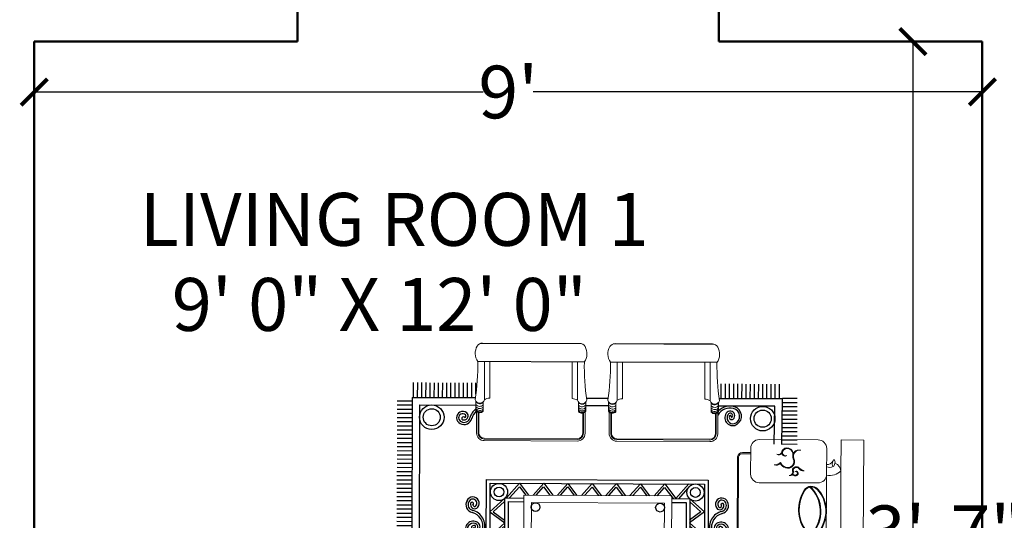
# Model space of a CAD drawing. Units: inches. Extents: x 147 to 1638, y 107 to 941.
# Tile 4 of 17: x 357 to 469, y 341 to 398. Entities that reach past the tile are written whole.
import ezdxf

# ---------------------------------------------------------------- set-up
doc = ezdxf.new("R2010")
doc.units = ezdxf.units.IN
doc.header["$MEASUREMENT"] = 0
for name, color, linetype, lineweight in [('A-ANNO-DIMS', 2, 'Continuous', 15), ('A-AREA-IDEN', 7, 'Continuous', 18), ('furniture', 50, 'Continuous', 18), ('wall', 7, 'Continuous', 60), ('walls', 7, 'Continuous', 50)]:
    doc.layers.add(name, color=color, linetype=linetype, lineweight=lineweight)
doc.layers.add('CARPET', color=40, linetype='Continuous')
doc.styles.get("Standard").update_dxf_attribs({"font": 'arial.ttf'})
doc.dimstyles.get("Standard").update_dxf_attribs({"dimtxt": 6, "dimasz": 3, "dimexe": 0.18, "dimexo": 0.0625, "dimgap": 0.09, "dimtad": 0, "dimtih": 1, "dimtoh": 1, "dimdec": 1, "dimzin": 0, "dimdsep": 46, "dimlunit": 3, "dimtxsty": 'Standard', "dimblk": 'ARCHTICK', "dimcen": 0.09, "dimadec": 0, "dimazin": 0, "dimtfac": 1, "dimtdec": 1, "dimtofl": 0, "dimtmove": 0, "dimatfit": 3, "dimfxl": 1, "dimtolj": 1, "dimtzin": 0, "dimarcsym": 0})

# ---------------------------------------------------------------- blocks, each defined once
blk = doc.blocks.new('_ArchTick')
at = {"color": 0, "linetype": 'ByBlock', "const_width": 0.15}
blk.add_lwpolyline([(-0.5, -0.5), (0.5, 0.5)], dxfattribs=at)
blk = doc.blocks.new('*D30')
at = {"layer": 'A-ANNO-DIMS', "color": 0, "lineweight": -2, "transparency": 16777216}
for p, q in [((460.3, 395.72), (458.86, 395.72)), ((459.04, 395.72), (459.04, 326.82)), ((459.04, 251.72), (459.04, 320.62)), ((460.3, 251.72), (458.86, 251.72))]:
    blk.add_line(p, q, dxfattribs=at)
at = {"layer": 'Defpoints', "color": 0, "lineweight": -2, "transparency": 16777216}
for p in [(460.36, 395.72), (459.04, 251.72), (460.36, 251.72)]:
    blk.add_point(p, dxfattribs=at)
at = {"layer": 'A-ANNO-DIMS', "color": 0, "lineweight": -2, "transparency": 16777216, "xscale": 3, "yscale": 3, "zscale": 3}
for p, rotation in [((459.04, 395.72), 90), ((459.04, 251.72), 270)]:
    blk.add_blockref('_ArchTick', p, dxfattribs=dict(at, rotation=rotation))
at = {"layer": 'A-ANNO-DIMS', "color": 0, "transparency": 16777216, "insert": (459.04, 323.72), "char_height": 6, "attachment_point": 5}
blk.add_mtext("\\A1;12'", dxfattribs=at)
blk = doc.blocks.new('*D31')
at = {"layer": 'A-ANNO-DIMS', "color": 0, "lineweight": -2, "transparency": 16777216}
for p, q in [((358.94, 390.58), (358.94, 389.8)), ((466.94, 390.58), (466.94, 389.8)), ((358.94, 389.98), (410.09, 389.98)), ((466.94, 389.98), (415.79, 389.98))]:
    blk.add_line(p, q, dxfattribs=at)
at = {"layer": 'Defpoints', "color": 0, "lineweight": -2, "transparency": 16777216}
for p in [(358.94, 390.65), (466.94, 390.65), (358.94, 389.98)]:
    blk.add_point(p, dxfattribs=at)
at = {"layer": 'A-ANNO-DIMS', "color": 0, "lineweight": -2, "transparency": 16777216, "xscale": 3, "yscale": 3, "zscale": 3, "rotation": 180}
blk.add_blockref('_ArchTick', (358.94, 389.98), dxfattribs=at)
at = {"layer": 'A-ANNO-DIMS', "color": 0, "lineweight": -2, "transparency": 16777216, "xscale": 3, "yscale": 3, "zscale": 3}
blk.add_blockref('_ArchTick', (466.94, 389.98), dxfattribs=at)
at = {"layer": 'A-ANNO-DIMS', "color": 0, "transparency": 16777216, "insert": (412.94, 389.98), "char_height": 6, "attachment_point": 5}
blk.add_mtext("\\A1;9'", dxfattribs=at)
blk = doc.blocks.new('X')
at = {"layer": 'furniture'}
for p, q in [((619.5149, -248.9209), (619.5149, -248.7654)), ((619.5149, -248.7654), (621.0036, -248.7654)), ((621.0036, -248.9205), (621.0036, -248.765)), ((619.5149, -248.9209), (619.7322, -248.9205)), ((619.7322, -248.9205), (620.6015, -248.9205)), ((621.0036, -248.9205), (620.6015, -248.9205)), ((619.5742, -249.0193), (619.752, -249.0193)), ((619.752, -249.0193), (620.6015, -249.0193)), ((620.2516, -249.5725), (620.2516, -249.0193)), ((620.259, -249.5725), (620.259, -249.0193)), ((620.259, -249.5725), (620.259, -249.0193)), ((620.2664, -249.5725), (620.2664, -249.0193)), ((620.9439, -249.0193), (620.6015, -249.0193)), ((619.5149, -249.0786), (619.5149, -249.4824)), ((619.8112, -249.4824), (619.8112, -249.0786)), ((620.7068, -249.4824), (620.7068, -249.0786)), ((621.0032, -249.4824), (621.0032, -249.0786)), ((619.5742, -249.5417), (619.752, -249.5417)), ((619.6049, -249.5417), (619.6049, -249.5987)), ((619.6124, -249.5417), (619.6124, -249.599)), ((620.9439, -249.5417), (620.7661, -249.5417)), ((620.9057, -249.5417), (620.9057, -249.599)), ((620.9131, -249.5417), (620.9131, -249.5987)), ((619.6334, -249.6243), (620.1998, -249.6243)), ((619.6334, -249.6317), (620.1998, -249.6317)), ((620.8846, -249.6243), (620.3183, -249.6243)), ((620.8846, -249.6317), (620.3183, -249.6317))]:
    blk.add_line(p, q, dxfattribs=at)
for centre, radius, start, end in [((619.7322, -248.9798), 0.0593, 90, 162.494), ((619.6556, -248.9979), 0.1044, 348.14652, 47.53007), ((620.8625, -248.9979), 0.1044, 132.46993, 191.85348), ((620.7859, -248.9798), 0.0593, 17.506, 90), ((619.635, -249.0188), 0.0496, 359.41182, 58.40348), ((619.6525, -249.0006), 0.0512, 338.60223, 29.59056), ((620.8656, -249.0006), 0.0512, 150.40944, 201.39777), ((620.8831, -249.0188), 0.0496, 121.59652, 180.58818), ((619.5742, -249.0786), 0.0593, 90, 180), ((619.752, -249.0786), 0.0593, 0, 90), ((620.007, -249.2904), 0.2333, 46.53167, 137.57273), ((620.007, -249.2904), 0.2283, 45.74065, 138.43075), ((620.007, -249.2476), 0.2283, 52.96969, 132.32477), ((620.007, -249.2476), 0.2234, 52.96969, 132.32477), ((620.1088, -249.1127), 0.0543, 307.98154, 52.96969), ((620.1088, -249.1127), 0.0593, 307.98154, 52.96969), ((620.4092, -249.1127), 0.0593, 127.03031, 232.01846), ((620.5111, -249.2904), 0.2333, 42.42727, 133.46833), ((620.5111, -249.2904), 0.2283, 41.56925, 134.25935), ((620.4092, -249.1127), 0.0543, 127.03031, 232.01846), ((620.5111, -249.2476), 0.2283, 47.67523, 127.03031), ((620.5111, -249.2476), 0.2234, 47.67523, 127.03031), ((620.7661, -249.0786), 0.0593, 90, 180), ((620.9439, -249.0786), 0.0593, 0, 90), ((619.8932, -249.1226), 0.0593, 132.32477, 237.31292), ((619.8932, -249.1226), 0.0543, 132.32477, 237.31292), ((620.6249, -249.1226), 0.0543, 302.68708, 47.67523), ((620.6249, -249.1226), 0.0593, 302.68708, 47.67523), ((619.6274, -249.2105), 0.0421, 161.95623, 295.85894), ((619.628, -249.2055), 0.0415, 168.85347, 291.99707), ((619.7278, -249.227), 0.0274, 132.99292, 265.5491), ((619.7278, -249.227), 0.0225, 132.99292, 262.0854), ((619.6678, -249.1626), 0.0605, 312.99292, 349.19232), ((619.6905, -249.1804), 0.0373, 306.00619, 9.85592), ((619.994, -248.9656), 0.2459, 237.31292, 307.98154), ((619.994, -248.9656), 0.241, 237.31292, 307.98154), ((620.5241, -248.9656), 0.2459, 232.01846, 302.68708), ((620.5241, -248.9656), 0.241, 232.01846, 302.68708), ((620.8276, -249.1804), 0.0373, 170.14408, 233.99381), ((620.8503, -249.1626), 0.0605, 190.80768, 227.00708), ((620.7903, -249.227), 0.0274, 274.4509, 47.00708), ((620.7903, -249.227), 0.0225, 277.9146, 47.00708), ((620.8907, -249.2105), 0.0421, 244.14106, 18.04377), ((620.89, -249.2055), 0.0415, 248.00293, 11.14653), ((619.6105, -249.2907), 0.0399, 81.34647, 244.80036), ((619.6138, -249.2892), 0.0378, 78.82007, 241.2356), ((619.6641, -249.2863), 0.0471, 341.95623, 115.85894), ((619.6641, -249.2863), 0.0421, 341.95623, 115.85894), ((619.7361, -249.2716), 0.0251, 55.31815, 117.0875), ((619.7357, -249.2774), 0.0252, 3.68155, 113.53579), ((619.745, -249.2275), 0.014, 61.30612, 229.17278), ((619.7459, -249.2313), 0.0122, 73.4413, 214.10415), ((619.7406, -249.2356), 0.0182, 302.61304, 61.30612), ((619.7406, -249.2356), 0.0232, 306.28248, 61.30612), ((619.7361, -249.2716), 0.0251, 350.3606, 43.63947), ((620.7775, -249.2356), 0.0232, 118.69388, 233.71752), ((620.782, -249.2716), 0.0251, 136.36053, 189.6394), ((620.7824, -249.2774), 0.0252, 66.46421, 176.31845), ((620.7775, -249.2356), 0.0182, 118.69388, 237.38696), ((620.7731, -249.2275), 0.014, 310.82722, 118.69388), ((620.782, -249.2716), 0.0251, 62.9125, 124.68185), ((620.7722, -249.2313), 0.0122, 325.89585, 106.5587), ((620.854, -249.2863), 0.0471, 64.14106, 198.04377), ((620.854, -249.2863), 0.0421, 64.14106, 198.04377), ((620.9043, -249.2892), 0.0378, 298.7644, 101.17993), ((620.9076, -249.2907), 0.0399, 295.19964, 98.65353), ((619.5921, -249.3513), 0.0246, 333.67342, 86.7751), ((619.6028, -249.3007), 0.0227, 251.57956, 22.48814), ((619.6037, -249.3051), 0.024, 287.88795, 33.0148), ((619.5947, -249.3467), 0.0249, 321.27483, 48.99439), ((619.6438, -249.2797), 0.0635, 295.85894, 341.95623), ((619.6335, -249.3751), 0.0539, 355.27866, 45.25264), ((619.6438, -249.2797), 0.0684, 298.77648, 341.95623), ((619.6593, -249.3656), 0.0313, 333.5007, 56.06813), ((620.8743, -249.2797), 0.0684, 198.04377, 241.22352), ((620.8743, -249.2797), 0.0635, 198.04377, 244.14106), ((620.8588, -249.3656), 0.0313, 123.93187, 206.4993), ((620.8845, -249.3751), 0.0539, 134.74736, 184.72134), ((620.9144, -249.3051), 0.024, 146.9852, 252.11205), ((620.9153, -249.3007), 0.0227, 157.51186, 288.42044), ((620.9233, -249.3467), 0.0249, 131.00561, 218.72517), ((620.926, -249.3513), 0.0246, 93.2249, 206.32658), ((619.5742, -249.4824), 0.0593, 180, 270), ((619.752, -249.4824), 0.0593, 270, 0), ((620.7661, -249.4824), 0.0593, 180, 270), ((620.9439, -249.4824), 0.0593, 270, 0), ((619.6387, -249.5984), 0.0338, 180.54468, 260.99104), ((619.6384, -249.5987), 0.0261, 179.37819, 258.97154), ((620.1998, -249.5725), 0.0593, 270, 0), ((620.1998, -249.5725), 0.0519, 270, 0), ((620.3183, -249.5725), 0.0593, 180, 270), ((620.3183, -249.5725), 0.0519, 180, 270), ((620.8796, -249.5987), 0.0261, 281.02846, 0.62181), ((620.8793, -249.5984), 0.0338, 279.00896, 359.45532)]:
    blk.add_arc(centre, radius, start, end, dxfattribs=at)
blk.add_ellipse((619.6743, -248.9709), major_axis=(-0.023, 0.0035), ratio=0.388107, start_param=3.141593, end_param=9.424778, dxfattribs=at)
at = {"layer": 'furniture', "extrusion": (0, 0, -1)}
blk.add_ellipse((620.8437, -248.9709), major_axis=(0.023, 0.0035), ratio=0.388107, start_param=3.141593, end_param=9.424778, dxfattribs=at)
blk = doc.blocks.new('sitting')
at = {"layer": 'CARPET'}
for p, q in [((0.3744, 0.8151), (0.3749, 0.9167)), ((0.403, 0.815), (0.4035, 0.9166)), ((0.4316, 0.8149), (0.432, 0.9165)), ((0.4602, 0.8148), (0.4606, 0.9164)), ((0.4887, 0.8147), (0.4892, 0.9163)), ((0.5173, 0.8145), (0.5178, 0.9161)), ((0.5459, 0.8144), (0.5463, 0.916)), ((0.5745, 0.8143), (0.5749, 0.9159)), ((0.603, 0.8142), (0.6035, 0.9158)), ((0.6316, 0.8141), (0.632, 0.9156)), ((0.6602, 0.8139), (0.6606, 0.9155)), ((0.6888, 0.8138), (0.6892, 0.9154)), ((2.1553, 0.8075), (2.1557, 0.9091)), ((2.1839, 0.8074), (2.1843, 0.909)), ((2.2125, 0.8073), (2.2129, 0.9089)), ((2.241, 0.8072), (2.2415, 0.9088)), ((2.2696, 0.8071), (2.27, 0.9087)), ((2.2982, 0.8069), (2.2986, 0.9085)), ((2.3268, 0.8068), (2.3272, 0.9084)), ((2.3553, 0.8067), (2.3558, 0.9083)), ((2.4603, 0.8998), (2.359, 0.9003)), ((0.3793, 0.8151), (0.3774, 0.3798)), ((0.6912, 0.81), (0.3793, 0.8151)), ((0.4301, 0.8149), (0.4301, 0.8143)), ((2.4599, 0.8141), (2.3586, 0.8145)), ((2.46, 0.8427), (2.3588, 0.8431)), ((2.4602, 0.8713), (2.3589, 0.8717)), ((0.379, 0.7658), (0.2774, 0.7663)), ((0.3791, 0.7944), (0.2775, 0.7949)), ((0.3791, 0.7643), (0.3785, 0.7643)), ((0.4299, 0.7635), (0.4282, 0.3764)), ((0.6904, 0.7592), (0.4299, 0.7635)), ((2.3073, 0.7561), (2.1474, 0.7568)), ((2.3583, 0.8067), (2.1476, 0.8076)), ((2.2981, -1.3815), (2.3073, 0.7561)), ((2.349, -1.3602), (2.3583, 0.8067)), ((2.4597, 0.757), (2.3584, 0.7574)), ((2.4598, 0.7855), (2.3585, 0.786)), ((0.3786, 0.6801), (0.277, 0.6806)), ((0.3788, 0.7087), (0.2772, 0.7091)), ((0.3789, 0.7373), (0.2773, 0.7377)), ((2.4594, 0.6998), (2.3582, 0.7002)), ((2.4596, 0.7284), (2.3583, 0.7288)), ((0.3784, 0.623), (0.2768, 0.6234)), ((0.3785, 0.6515), (0.2769, 0.652)), ((2.4591, 0.6141), (2.3578, 0.6145)), ((2.4592, 0.6427), (2.3579, 0.6431)), ((2.4593, 0.6712), (2.358, 0.6717)), ((0.3782, 0.5658), (0.2766, 0.5663)), ((0.3783, 0.5944), (0.2767, 0.5948)), ((2.4588, 0.5569), (2.3576, 0.5574)), ((2.4589, 0.5855), (2.3577, 0.586)), ((0.3778, 0.4801), (0.2762, 0.4805)), ((0.3779, 0.5087), (0.2763, 0.5091)), ((0.378, 0.5372), (0.2764, 0.5377)), ((2.4586, 0.4998), (2.3573, 0.5002)), ((2.4587, 0.5284), (2.3574, 0.5288)), ((0.3775, 0.4229), (0.2759, 0.4234)), ((0.3777, 0.4515), (0.2761, 0.452)), ((2.4582, 0.4141), (2.3569, 0.4145)), ((2.4583, 0.4426), (2.3571, 0.4431)), ((2.4585, 0.4712), (2.3572, 0.4717)), ((0.3774, 0.3944), (0.2758, 0.3948)), ((2.458, 0.3569), (2.3567, 0.3574)), ((2.4581, 0.3855), (2.3568, 0.3859)), ((1.065, 0.178), (1.1552, 0.2792)), ((1.1552, 0.2792), (1.2313, 0.1773)), ((1.2313, 0.1773), (1.3215, 0.2785)), ((1.3215, 0.2785), (1.3976, 0.1766)), ((1.3976, 0.1766), (1.4877, 0.2778)), ((1.4877, 0.2778), (1.5638, 0.1759)), ((2.4576, 0.2712), (2.3563, 0.2716)), ((2.4577, 0.2998), (2.3565, 0.3002)), ((2.4578, 0.3283), (2.3566, 0.3288)), ((1.0854, 0.1779), (1.1542, 0.2552)), ((1.1542, 0.2552), (1.2122, 0.1774)), ((1.2516, 0.1772), (1.3204, 0.2544)), ((1.3204, 0.2544), (1.3785, 0.1767)), ((1.4179, 0.1765), (1.4867, 0.2537)), ((1.4867, 0.2537), (1.5447, 0.176)), ((1.5638, 0.1759), (1.5928, 0.2111)), ((2.4574, 0.214), (2.3561, 0.2145)), ((2.4575, 0.2426), (2.3562, 0.2431)), ((1.0646, 0.0827), (0.9634, 0.1728)), ((1.0647, 0.103), (0.9951, 0.165)), ((1.6077, 0.0803), (1.7096, 0.1696)), ((1.6077, 0.1007), (1.6779, 0.1621)), ((1.7096, 0.1696), (1.6979, 0.1786)), ((2.4571, 0.1569), (2.3558, 0.1573)), ((2.4572, 0.1855), (2.356, 0.1859)), ((0.9627, 0.0066), (1.0646, 0.0827)), ((1.6441, 0.0527), (1.6077, 0.0803)), ((2.4567, 0.0712), (2.3555, 0.0716)), ((2.4569, 0.0997), (2.3556, 0.1002)), ((2.457, 0.1283), (2.3557, 0.1288)), ((1.0444, -0.0662), (0.9627, 0.0066)), ((0.9868, 0.0055), (1.0646, 0.0636)), ((1.0444, -0.0458), (0.9868, 0.0055)), ((1.6188, 0.0528), (1.6076, 0.0613)), ((1.6859, -0.0168), (1.7089, 0.0034)), ((1.7089, 0.0034), (1.6861, 0.0207)), ((2.4565, 0.014), (2.3552, 0.0145)), ((2.4566, 0.0426), (2.3554, 0.043)), ((2.4563, -0.0431), (2.355, -0.0427)), ((2.4564, -0.0146), (2.3551, -0.0141)), ((0.962, -0.1597), (1.0442, -0.0983)), ((0.9861, -0.1607), (1.0441, -0.1174)), ((2.4559, -0.1288), (2.3546, -0.1284)), ((2.456, -0.1003), (2.3547, -0.0998)), ((2.4561, -0.0717), (2.3549, -0.0713)), ((1.0436, -0.2324), (0.962, -0.1597)), ((1.0437, -0.2121), (0.9861, -0.1607)), ((1.6852, -0.183), (1.7082, -0.1629)), ((1.7082, -0.1629), (1.6854, -0.1455)), ((2.4557, -0.186), (2.3544, -0.1856)), ((2.4558, -0.1574), (2.3545, -0.157)), ((0.9613, -0.326), (1.0435, -0.2646)), ((2.4554, -0.2431), (2.3541, -0.2427)), ((2.4555, -0.2146), (2.3543, -0.2141)), ((1.0429, -0.3987), (0.9613, -0.326)), ((0.9854, -0.327), (1.0434, -0.2837)), ((1.043, -0.3784), (0.9854, -0.327)), ((1.6845, -0.3493), (1.7075, -0.3291)), ((1.7075, -0.3291), (1.6847, -0.3118)), ((2.455, -0.3289), (2.3538, -0.3284)), ((2.4552, -0.3003), (2.3539, -0.2999)), ((2.4553, -0.2717), (2.354, -0.2713)), ((0.3734, -0.5318), (0.374, -0.383)), ((0.4242, -0.5353), (0.4248, -0.38)), ((2.4548, -0.386), (2.3535, -0.3856)), ((2.4549, -0.3574), (2.3537, -0.357)), ((0.9606, -0.4922), (1.0428, -0.4308)), ((0.9847, -0.4933), (1.0427, -0.4499)), ((2.4544, -0.4717), (2.3532, -0.4713)), ((2.4546, -0.4432), (2.3533, -0.4427)), ((2.4547, -0.4146), (2.3534, -0.4142)), ((1.0422, -0.5649), (0.9606, -0.4922)), ((1.0423, -0.5446), (0.9847, -0.4933)), ((1.6838, -0.5155), (1.7068, -0.4954)), ((1.7068, -0.4954), (1.684, -0.478)), ((2.4542, -0.5289), (2.3529, -0.5285)), ((2.4543, -0.5003), (2.353, -0.4999)), ((0.9599, -0.6585), (1.0421, -0.5971)), ((2.4539, -0.586), (2.3527, -0.5856)), ((2.4541, -0.5575), (2.3528, -0.557)), ((1.0415, -0.7312), (0.9599, -0.6585)), ((0.984, -0.6595), (1.042, -0.6162)), ((1.0416, -0.7109), (0.984, -0.6595)), ((1.6831, -0.6818), (1.7061, -0.6617)), ((1.7061, -0.6617), (1.6833, -0.6443)), ((2.4536, -0.6718), (2.3523, -0.6713)), ((2.4537, -0.6432), (2.3524, -0.6428)), ((2.4538, -0.6146), (2.3526, -0.6142)), ((2.4533, -0.7289), (2.3521, -0.7285)), ((2.4535, -0.7003), (2.3522, -0.6999)), ((0.9592, -0.8247), (1.0414, -0.7634)), ((0.9832, -0.8258), (1.0413, -0.7824)), ((1.7054, -0.8279), (1.6825, -0.8106)), ((2.4531, -0.7861), (2.3518, -0.7856)), ((2.4532, -0.7575), (2.3519, -0.7571)), ((1.0408, -0.8975), (0.9592, -0.8247)), ((1.0409, -0.8771), (0.9832, -0.8258)), ((1.6824, -0.8481), (1.7054, -0.8279)), ((2.4527, -0.8718), (2.3515, -0.8714)), ((2.4528, -0.8432), (2.3516, -0.8428)), ((2.453, -0.8146), (2.3517, -0.8142)), ((0.9585, -0.991), (1.0407, -0.9296)), ((2.4525, -0.9289), (2.3512, -0.9285)), ((2.4526, -0.9004), (2.3513, -0.8999)), ((1.0597, -1.0812), (0.9585, -0.991)), ((0.9825, -0.992), (1.0406, -0.9487)), ((1.0598, -1.0608), (0.9825, -0.992)), ((1.6027, -1.0835), (1.7047, -0.9942)), ((1.6028, -1.0632), (1.6806, -0.995)), ((1.6806, -0.995), (1.6392, -0.9636)), ((1.7047, -0.9942), (1.6645, -0.9637)), ((2.4521, -1.0147), (2.3508, -1.0142)), ((2.4522, -0.9861), (2.351, -0.9857)), ((2.4524, -0.9575), (2.3511, -0.9571)), ((2.4519, -1.0718), (2.3506, -1.0714)), ((2.452, -1.0432), (2.3507, -1.0428)), ((1.0645, -1.0959), (1.1557, -1.1962)), ((1.0848, -1.0956), (1.1544, -1.1721)), ((1.1544, -1.1721), (1.2117, -1.0938)), ((1.1557, -1.1962), (1.2307, -1.0935)), ((1.2307, -1.0935), (1.3219, -1.1938)), ((1.2511, -1.0932), (1.3206, -1.1697)), ((1.3206, -1.1697), (1.3779, -1.0914)), ((1.3219, -1.1938), (1.397, -1.0911)), ((1.397, -1.0911), (1.4882, -1.1914)), ((1.4173, -1.0908), (1.4869, -1.1674)), ((1.4869, -1.1674), (1.5442, -1.089)), ((1.4882, -1.1914), (1.5632, -1.0887)), ((1.5632, -1.0887), (1.5926, -1.1237)), ((2.4516, -1.129), (2.3504, -1.1285)), ((2.4517, -1.1004), (2.3505, -1.1)), ((2.4513, -1.2147), (2.35, -1.2143)), ((2.4514, -1.1861), (2.3501, -1.1857)), ((2.4515, -1.1575), (2.3502, -1.1571)), ((2.451, -1.2718), (2.3498, -1.2714)), ((2.4511, -1.2433), (2.3499, -1.2428)), ((0.37, -1.3487), (0.2684, -1.3483)), ((0.3701, -1.3201), (0.2685, -1.3197)), ((0.3458, -1.2914), (0.2686, -1.2911)), ((0.3684, -1.73), (0.3702, -1.2947)), ((0.4194, -1.6792), (0.421, -1.2917)), ((2.4508, -1.329), (2.3495, -1.3286)), ((2.4509, -1.3004), (2.3496, -1.3)), ((0.3697, -1.4058), (0.2681, -1.4054)), ((0.3699, -1.3773), (0.2683, -1.3768)), ((2.4507, -1.3576), (2.3494, -1.3571)), ((2.4505, -1.3861), (2.3623, -1.3858)), ((2.4504, -1.4147), (2.3793, -1.4144)), ((0.3695, -1.463), (0.2679, -1.4626)), ((0.3696, -1.4344), (0.268, -1.434)), ((2.4503, -1.4433), (2.3989, -1.4431)), ((2.4502, -1.4719), (2.4215, -1.4717)), ((0.3691, -1.5487), (0.2675, -1.5483)), ((0.3693, -1.5201), (0.2677, -1.5197)), ((0.3694, -1.4916), (0.2678, -1.4911)), ((0.3689, -1.6059), (0.2673, -1.6054)), ((0.369, -1.5773), (0.2674, -1.5769)), ((0.3685, -1.6916), (0.2669, -1.6912)), ((0.3686, -1.663), (0.267, -1.6626)), ((0.3688, -1.6344), (0.2672, -1.634)), ((0.3685, -1.6792), (0.3686, -1.6792)), ((0.4194, -1.6792), (1.9199, -1.6809)), ((2.2497, -1.6758), (2.2797, -1.7508)), ((2.2561, -1.6735), (2.2901, -1.7588)), ((2.2845, -1.6663), (2.3262, -1.7708)), ((2.2896, -1.6655), (2.3296, -1.7657)), ((2.2995, -1.6644), (2.3358, -1.7553)), ((2.3112, -1.6637), (2.3424, -1.7417)), ((0.3684, -1.7202), (0.2668, -1.7197)), ((0.3684, -1.73), (1.8242, -1.7316)), ((0.3917, -1.8317), (0.3922, -1.7301)), ((0.4203, -1.8318), (0.4207, -1.7302)), ((0.4489, -1.8319), (0.4493, -1.7303)), ((0.4775, -1.832), (0.4779, -1.7304)), ((0.506, -1.8322), (0.5065, -1.7306)), ((0.5346, -1.8323), (0.535, -1.7307)), ((0.5632, -1.8324), (0.5636, -1.7308)), ((0.5917, -1.8325), (0.5922, -1.7309)), ((0.6203, -1.8327), (0.6208, -1.7311)), ((0.6489, -1.8328), (0.6493, -1.7312)), ((0.6775, -1.8329), (0.6779, -1.7313)), ((0.6775, -1.8329), (0.6779, -1.7313)), ((0.706, -1.833), (0.7065, -1.7314)), ((0.7346, -1.8331), (0.7351, -1.7315)), ((0.7632, -1.8333), (0.7636, -1.7317)), ((0.7918, -1.8334), (0.7922, -1.7318)), ((0.8203, -1.8335), (0.8208, -1.7319)), ((0.8489, -1.8336), (0.8494, -1.732)), ((0.8775, -1.8338), (0.8779, -1.7322)), ((0.9061, -1.8339), (0.9065, -1.7323)), ((0.9346, -1.834), (0.9351, -1.7324)), ((0.9632, -1.8341), (0.9637, -1.7325)), ((0.9632, -1.8341), (0.9637, -1.7325)), ((0.9918, -1.8342), (0.9922, -1.7326)), ((1.0204, -1.8344), (1.0208, -1.7328)), ((1.0489, -1.8345), (1.0494, -1.7329)), ((1.0775, -1.8346), (1.078, -1.733)), ((1.1061, -1.8347), (1.1065, -1.7331)), ((1.1347, -1.8349), (1.1351, -1.7333)), ((1.1632, -1.835), (1.1637, -1.7334)), ((1.1918, -1.8351), (1.1923, -1.7335)), ((1.2204, -1.8352), (1.2208, -1.7336)), ((1.249, -1.8353), (1.2494, -1.7337)), ((1.249, -1.8353), (1.2494, -1.7337)), ((1.2775, -1.8355), (1.278, -1.7339)), ((1.3061, -1.8356), (1.3066, -1.734)), ((1.3347, -1.8357), (1.3351, -1.7341)), ((1.3633, -1.8358), (1.3637, -1.7342)), ((1.3918, -1.8359), (1.3923, -1.7344)), ((1.4204, -1.8361), (1.4209, -1.7345)), ((1.449, -1.8362), (1.4494, -1.7346)), ((1.4776, -1.8363), (1.478, -1.7347)), ((1.5061, -1.8364), (1.5066, -1.7348)), ((1.5347, -1.8366), (1.5351, -1.735)), ((1.5347, -1.8366), (1.5351, -1.735)), ((1.5633, -1.8367), (1.5637, -1.7351)), ((1.5919, -1.8368), (1.5923, -1.7352)), ((1.6204, -1.8369), (1.6209, -1.7353)), ((1.649, -1.837), (1.6494, -1.7354)), ((1.6776, -1.8372), (1.678, -1.7356)), ((1.7062, -1.8373), (1.7066, -1.7357)), ((1.7347, -1.8374), (1.7352, -1.7358)), ((1.7633, -1.8375), (1.7637, -1.7359)), ((1.7919, -1.8377), (1.7923, -1.7361)), ((1.8205, -1.8378), (1.8209, -1.7362)), ((1.8205, -1.8378), (1.8209, -1.7362)), ((1.8776, -1.838), (1.878, -1.7463)), ((1.9062, -1.8381), (1.9065, -1.7539)), ((2.1669, -1.7607), (2.2209, -1.7306)), ((2.1682, -1.7716), (2.2377, -1.7329)), ((2.1696, -1.7798), (2.2486, -1.7358)), ((2.1767, -1.8083), (2.2798, -1.7509)), ((2.1869, -1.7158), (2.1934, -1.732)), ((2.1905, -1.7124), (2.1981, -1.7313)), ((2.1949, -1.7086), (2.2037, -1.7307)), ((2.2165, -1.6925), (2.2322, -1.7319)), ((2.3154, -1.7846), (2.4341, -1.7427)), ((2.3177, -1.7875), (2.4393, -1.7513)), ((2.3392, -1.7487), (2.4162, -1.7184)), ((2.3496, -1.7218), (2.4007, -1.7017)), ((2.3514, -1.7152), (2.3825, -1.7029)), ((2.353, -1.7075), (2.3836, -1.6955)), ((1.849, -1.8379), (1.8494, -1.7604)), ((1.9348, -1.8383), (1.935, -1.7772)), ((1.9348, -1.8383), (1.935, -1.7772)), ((1.9633, -1.8384), (1.9635, -1.8042)), ((2.1854, -1.8315), (2.2996, -1.7679)), ((2.1876, -1.8364), (2.3032, -1.7719)), ((2.1988, -1.8576), (2.3106, -1.7953)), ((2.2023, -1.8633), (2.3072, -1.8049)), ((2.2069, -1.8702), (2.3018, -1.8173)), ((2.3011, -1.8189), (2.3211, -1.9184)), ((2.3067, -1.8053), (2.3293, -1.9175)), ((2.3142, -1.7864), (2.3404, -1.9165)), ((2.3375, -1.7853), (2.3628, -1.9109)), ((2.3403, -1.7854), (2.3836, -1.7684)), ((2.3425, -1.7855), (2.3676, -1.9096)), ((2.3667, -1.7885), (2.3896, -1.9022)), ((2.3849, -1.7941), (2.4485, -1.7704)), ((2.3952, -1.797), (2.4141, -1.8911)), ((2.3975, -1.7979), (2.448, -1.7755)), ((2.4068, -1.802), (2.4237, -1.8859)), ((2.2731, -1.8735), (2.2823, -1.919)), ((2.297, -1.8281), (2.3153, -1.9188))]:
    blk.add_line(p, q, dxfattribs=at)
for points in [[(0.9321, -1.2188), (0.9386, 0.3056), (1.7356, 0.3022), (1.7291, -1.2222)], [(0.9576, -1.1935), (0.9639, 0.2801), (1.7101, 0.2769), (1.7038, -1.1967)]]:
    blk.add_lwpolyline(points, close=True, dxfattribs=at)
for points in [[(1.0645, 0.0551), (1.065, 0.178), (1.6081, 0.1757), (1.6075, 0.0528)], [(1.0899, 0.055), (1.0903, 0.1525), (1.5826, 0.1504), (1.5821, 0.0529)], [(1.6032, -0.9634), (1.6026, -1.0947), (1.0596, -1.0923), (1.0602, -0.9611)], [(1.5778, -0.9633), (1.5774, -1.0692), (1.0851, -1.0671), (1.0856, -0.9612)]]:
    blk.add_lwpolyline(points, dxfattribs=at)
for centre, radius in [((0.5147, 0.6796), 0.0843), ((2.2246, 0.6725), 0.0843), ((0.5147, 0.6796), 0.0589), ((2.2246, 0.6725), 0.0589), ((1.022, 0.2174), 0.0589), ((1.6516, 0.2147), 0.0589), ((1.022, 0.2174), 0.0335), ((1.6516, 0.2147), 0.0335), ((1.1262, -0.0259), 0.0301), ((1.6047, -0.028), 0.0301), ((1.1225, -0.881), 0.0301), ((1.601, -0.883), 0.0301), ((1.0184, -1.1325), 0.0589), ((1.6479, -1.1352), 0.0589), ((1.0184, -1.1325), 0.0335), ((1.6479, -1.1352), 0.0335), ((0.505, -1.5948), 0.0843), ((0.505, -1.5948), 0.0589)]:
    blk.add_circle(centre, radius, dxfattribs=at)
for centre, radius, start, end in [((0.5416, 0.4551), 0.1132, 163.72753, 224.16333), ((0.497, 0.4669), 0.067, 33.92326, 162.74749), ((0.5428, 0.4571), 0.1008, 166.99629, 238.96019), ((0.4977, 0.4665), 0.0548, 20.90664, 165.92882), ((0.4936, 0.4564), 0.0315, 41.04313, 239.89648), ((0.5086, 0.4733), 0.0538, 235.07981, 35.18035), ((0.5086, 0.4759), 0.0415, 235.36127, 14.07703), ((0.5048, 0.4662), 0.0166, 231.08782, 41.04313), ((2.2298, 0.466), 0.0538, 144.33076, 304.4313), ((2.2413, 0.4595), 0.067, 16.76363, 145.58785), ((2.2297, 0.4686), 0.0415, 165.43408, 304.14985), ((2.2406, 0.459), 0.0548, 13.58229, 158.60447), ((2.2447, 0.449), 0.0315, 299.61464, 138.46799), ((2.1966, 0.448), 0.1132, 284.45049, 15.78359), ((0.4936, 0.4564), 0.0169, 41.04313, 239.89648), ((0.5005, 0.4578), 0.00755, 65.8585, 269.29351), ((0.5048, 0.4662), 0.00198, 231.08782, 41.04313), ((1.1039, 0.3982), 0.0436, 112.88129, 307.21618), ((1.1031, 0.3985), 0.0284, 110.32478, 311.53076), ((1.1129, 0.3899), 0.055, 11.99051, 119.18067), ((1.1129, 0.3899), 0.0404, 11.99051, 119.18067), ((1.1077, 0.403), 0.011, 65.50738, 327.11735), ((1.1131, 0.3853), 0.0277, 308.26022, 91.73038), ((1.2799, 0.3933), 0.0538, 54.33076, 214.4313), ((1.2825, 0.3934), 0.0415, 75.43408, 214.14985), ((1.2728, 0.3896), 0.0166, 48.46799, 218.4233), ((1.273, 0.3825), 0.0548, 283.58229, 68.60447), ((1.2734, 0.3818), 0.067, 286.76363, 55.58785), ((1.4074, 0.3811), 0.067, 123.92326, 252.74749), ((1.4078, 0.3819), 0.0548, 110.90664, 255.92882), ((1.401, 0.3927), 0.0538, 325.07981, 125.18035), ((1.3984, 0.3928), 0.0415, 325.36127, 104.07703), ((1.5679, 0.3879), 0.055, 60.33045, 167.52061), ((1.5679, 0.3879), 0.0404, 60.33045, 167.52061), ((1.5677, 0.3833), 0.0277, 87.78073, 231.2509), ((1.577, 0.3961), 0.0436, 232.29494, 66.62983), ((1.5778, 0.3964), 0.0284, 227.98036, 69.18634), ((1.5733, 0.4009), 0.011, 212.39376, 114.00374), ((2.2335, 0.4588), 0.0166, 138.46799, 308.4233), ((2.1954, 0.45), 0.1008, 284.1961, 12.51483), ((2.2335, 0.4588), 0.00198, 138.46799, 308.4233), ((2.2447, 0.449), 0.0169, 299.61464, 138.46799), ((2.2377, 0.4504), 0.00755, 270.2176, 113.65261), ((1.1133, 0.3856), 0.012, 316.00944, 72.44807), ((1.262, 0.4266), 0.1132, 194.45049, 285.78359), ((1.264, 0.4277), 0.1008, 194.1961, 282.51483), ((1.2629, 0.3785), 0.0315, 209.61464, 48.46799), ((1.2629, 0.3785), 0.0169, 209.61464, 48.46799), ((1.2643, 0.3854), 0.00755, 180.2176, 23.65261), ((1.2728, 0.3896), 0.00198, 48.46799, 218.4233), ((1.4179, 0.3777), 0.0315, 131.04313, 329.89648), ((1.4192, 0.4258), 0.1132, 253.72753, 345.06062), ((1.4172, 0.4269), 0.1008, 256.99629, 345.31502), ((1.4081, 0.389), 0.0166, 321.08782, 131.04313), ((1.4179, 0.3777), 0.0169, 131.04313, 329.89648), ((1.4081, 0.389), 0.00198, 321.08782, 131.04313), ((1.4165, 0.3846), 0.00755, 155.8585, 359.29351), ((1.5675, 0.3835), 0.012, 107.06305, 223.50168), ((2.2332, 0.299), 0.055, 101.99051, 209.18067), ((2.2332, 0.299), 0.0404, 101.99051, 209.18067), ((2.2249, 0.29), 0.0436, 202.88129, 37.21618), ((2.2246, 0.2892), 0.0284, 200.32478, 41.53076), ((2.2201, 0.2937), 0.011, 155.50738, 57.11735), ((2.2378, 0.2991), 0.0277, 38.26022, 181.73038), ((2.2376, 0.2994), 0.012, 46.00944, 162.44807), ((2.2327, 0.1959), 0.055, 150.33045, 257.52061), ((2.2245, 0.205), 0.0436, 322.29494, 156.62983), ((2.2327, 0.1959), 0.0404, 150.33045, 257.52061), ((2.2243, 0.2058), 0.0284, 317.98036, 159.18634), ((2.2197, 0.2012), 0.011, 302.39376, 204.00374), ((2.2374, 0.1957), 0.0277, 177.78073, 321.2509), ((2.1937, 0.0451), 0.1008, 346.99629, 75.31502), ((2.1948, 0.0472), 0.1132, 343.72753, 75.06062), ((2.2371, 0.1955), 0.012, 197.06305, 313.50168), ((2.2279, 0.0289), 0.0538, 55.07981, 215.18035), ((2.2278, 0.0263), 0.0415, 55.36127, 194.07703), ((2.2429, 0.0458), 0.0315, 221.04313, 59.89648), ((2.2395, 0.0353), 0.067, 213.92326, 342.74749), ((2.2388, 0.0358), 0.0548, 200.90664, 345.92882), ((2.2317, 0.036), 0.0166, 51.08782, 221.04313), ((2.2317, 0.036), 0.00198, 51.08782, 221.04313), ((2.2429, 0.0458), 0.0169, 221.04313, 59.89648), ((2.236, 0.0445), 0.00755, 245.8585, 89.29351), ((2.2275, -0.0922), 0.0538, 144.33076, 304.4313), ((2.239, -0.0986), 0.067, 16.76363, 145.58785), ((2.2383, -0.0991), 0.0548, 13.58229, 158.60447), ((2.2274, -0.0895), 0.0415, 165.43408, 304.14985), ((2.2312, -0.0993), 0.0166, 138.46799, 308.4233), ((2.1931, -0.1081), 0.1008, 284.1961, 12.51483), ((2.2424, -0.1091), 0.0315, 299.61464, 138.46799), ((2.1942, -0.1101), 0.1132, 284.45049, 15.78359), ((2.2312, -0.0993), 0.00198, 138.46799, 308.4233), ((2.2424, -0.1091), 0.0169, 299.61464, 138.46799), ((2.2354, -0.1077), 0.00755, 270.2176, 113.65261), ((2.2309, -0.2591), 0.055, 101.99051, 209.18067), ((2.2226, -0.2681), 0.0436, 202.88129, 37.21618), ((2.2309, -0.2591), 0.0404, 101.99051, 209.18067), ((2.2223, -0.2689), 0.0284, 200.32478, 41.53076), ((2.2178, -0.2644), 0.011, 155.50738, 57.11735), ((2.2355, -0.259), 0.0277, 38.26022, 181.73038), ((2.2352, -0.2587), 0.012, 46.00944, 162.44807), ((2.2282, -0.3643), 0.055, 150.33045, 257.52061), ((2.22, -0.3553), 0.0436, 322.29494, 156.62983), ((2.2197, -0.3545), 0.0284, 317.98036, 159.18634), ((2.2282, -0.3643), 0.0404, 150.33045, 257.52061), ((2.2152, -0.359), 0.011, 302.39376, 204.00374), ((2.2328, -0.3646), 0.0277, 177.78073, 321.2509), ((2.1903, -0.5131), 0.1132, 343.72753, 75.06062), ((2.2326, -0.3648), 0.012, 197.06305, 313.50168), ((2.1892, -0.5151), 0.1008, 346.99629, 75.31502), ((2.2234, -0.5313), 0.0538, 55.07981, 215.18035), ((2.2233, -0.5339), 0.0415, 55.36127, 194.07703), ((2.2342, -0.5244), 0.0548, 200.90664, 345.92882), ((2.2276, -0.5255), 0.0166, 51.08782, 221.04313), ((2.2384, -0.5144), 0.0315, 221.04313, 59.89648), ((2.2384, -0.5144), 0.0169, 221.04313, 59.89648), ((2.2276, -0.5255), 0.00198, 51.08782, 221.04313), ((2.232, -0.5171), 0.00755, 245.8585, 89.29351), ((2.2345, -0.6588), 0.067, 16.76363, 145.58785), ((2.235, -0.5249), 0.067, 213.92326, 342.74749), ((2.2337, -0.6593), 0.0548, 13.58229, 158.60447), ((2.2229, -0.6524), 0.0538, 144.33076, 304.4313), ((2.2229, -0.6498), 0.0415, 165.43408, 304.14985), ((2.2271, -0.6608), 0.0166, 138.46799, 308.4233), ((2.1886, -0.6683), 0.1008, 284.1961, 12.51483), ((2.2378, -0.6694), 0.0315, 299.61464, 138.46799), ((2.1897, -0.6703), 0.1132, 284.45049, 15.78359), ((2.2378, -0.6694), 0.0169, 299.61464, 138.46799), ((2.2271, -0.6608), 0.00198, 138.46799, 308.4233), ((2.2314, -0.6693), 0.00755, 270.2176, 113.65261), ((2.2263, -0.8194), 0.055, 101.99051, 209.18067), ((2.218, -0.8284), 0.0436, 202.88129, 37.21618), ((2.2263, -0.8194), 0.0404, 101.99051, 209.18067), ((2.2177, -0.8292), 0.0284, 200.32478, 41.53076), ((2.2309, -0.8192), 0.0277, 38.26022, 181.73038), ((2.2307, -0.819), 0.012, 46.00944, 162.44807), ((2.216, -0.9155), 0.0436, 322.29494, 156.62983), ((2.2132, -0.8246), 0.011, 155.50738, 57.11735), ((2.2242, -0.9246), 0.055, 150.33045, 257.52061), ((2.2242, -0.9246), 0.0404, 150.33045, 257.52061), ((2.2157, -0.9147), 0.0284, 317.98036, 159.18634), ((2.2112, -0.9192), 0.011, 302.39376, 204.00374), ((2.2288, -0.9248), 0.0277, 177.78073, 321.2509), ((2.2286, -0.925), 0.012, 197.06305, 313.50168), ((2.1852, -1.0753), 0.1008, 346.99629, 75.31502), ((2.1863, -1.0733), 0.1132, 343.72753, 75.06062), ((2.2194, -1.0915), 0.0538, 55.07981, 215.18035), ((2.2193, -1.0941), 0.0415, 55.36127, 194.07703), ((2.2231, -1.0844), 0.0166, 51.08782, 221.04313), ((2.2344, -1.0746), 0.0315, 221.04313, 59.89648), ((2.2231, -1.0844), 0.00198, 51.08782, 221.04313), ((2.2344, -1.0746), 0.0169, 221.04313, 59.89648), ((2.2275, -1.076), 0.00755, 245.8585, 89.29351), ((2.231, -1.0852), 0.067, 213.92326, 342.74749), ((2.2302, -1.0847), 0.0548, 200.90664, 345.92882), ((2.2189, -1.2126), 0.0538, 144.33076, 304.4313), ((2.2305, -1.2191), 0.067, 16.76363, 145.58785), ((2.2189, -1.21), 0.0415, 165.43408, 304.14985), ((2.2297, -1.2195), 0.0548, 13.58229, 158.60447), ((2.2231, -1.221), 0.0166, 138.46799, 308.4233), ((2.1846, -1.2285), 0.1008, 284.1961, 12.51483), ((2.2338, -1.2296), 0.0315, 299.61464, 138.46799), ((2.1857, -1.2305), 0.1132, 284.45049, 15.78359), ((2.2338, -1.2296), 0.0169, 299.61464, 138.46799), ((1.0966, -1.3129), 0.0436, 52.29494, 246.62983), ((1.0958, -1.3131), 0.0284, 47.98036, 249.18634), ((1.1059, -1.3), 0.0277, 267.78073, 51.2509), ((1.2544, -1.3426), 0.1132, 73.72753, 165.06062), ((1.2564, -1.3437), 0.1008, 76.99629, 165.31502), ((1.2726, -1.3095), 0.0538, 145.07981, 305.18035), ((1.2558, -1.2945), 0.0315, 311.04313, 149.89648), ((1.2558, -1.2945), 0.0169, 311.04313, 149.89648), ((1.2658, -1.2986), 0.0548, 290.90664, 75.92882), ((1.2663, -1.2979), 0.067, 303.92326, 72.74749), ((1.4002, -1.2984), 0.067, 106.76363, 235.58785), ((1.4007, -1.2991), 0.0548, 103.58229, 248.60447), ((1.3937, -1.3099), 0.0538, 234.33076, 34.4313), ((1.4107, -1.295), 0.0315, 29.61464, 228.46799), ((1.4117, -1.3432), 0.1132, 14.45049, 105.78359), ((1.4096, -1.3443), 0.1008, 14.1961, 102.51483), ((1.4107, -1.295), 0.0169, 29.61464, 228.46799), ((1.5605, -1.3019), 0.0277, 128.26022, 271.73038), ((1.5697, -1.3148), 0.0436, 292.88129, 127.21618), ((2.2231, -1.221), 0.00198, 138.46799, 308.4233), ((2.2274, -1.2295), 0.00755, 270.2176, 113.65261), ((0.5381, -1.2235), 0.1132, 217.11392, 255.06062), ((0.5393, -1.2215), 0.1008, 221.67675, 255.31502), ((0.4956, -1.372), 0.0277, 357.78073, 141.2509), ((0.5002, -1.3723), 0.0404, 330.33045, 77.52061), ((0.5002, -1.3723), 0.055, 330.33045, 77.52061), ((1.1057, -1.3047), 0.055, 240.33045, 347.52061), ((1.1057, -1.3047), 0.0404, 240.33045, 347.52061), ((1.1003, -1.3177), 0.011, 32.39376, 294.00374), ((1.1061, -1.3003), 0.012, 287.06305, 43.50168), ((1.2753, -1.3096), 0.0415, 145.36127, 284.07703), ((1.2656, -1.3057), 0.0166, 141.08782, 311.04313), ((1.2571, -1.3014), 0.00755, 335.8585, 179.29351), ((1.2656, -1.3057), 0.00198, 141.08782, 311.04313), ((1.3911, -1.31), 0.0415, 255.43408, 34.14985), ((1.4008, -1.3062), 0.0166, 228.46799, 38.4233), ((1.4008, -1.3062), 0.00198, 228.46799, 38.4233), ((1.4093, -1.302), 0.00755, 0.2176, 203.65261), ((1.5607, -1.3065), 0.055, 191.99051, 299.18067), ((1.5607, -1.3065), 0.0404, 191.99051, 299.18067), ((1.5603, -1.3022), 0.012, 136.00944, 252.44807), ((1.5705, -1.3151), 0.0284, 290.32478, 131.53076), ((1.5659, -1.3196), 0.011, 245.50738, 147.11735), ((2.2223, -1.3796), 0.055, 101.99051, 209.18067), ((2.2223, -1.3796), 0.0404, 101.99051, 209.18067), ((2.2269, -1.3794), 0.0277, 38.26022, 181.73038), ((0.5085, -1.3813), 0.0436, 142.29494, 336.62983), ((0.5087, -1.3821), 0.0284, 137.98036, 339.18634), ((0.4959, -1.3718), 0.012, 17.06305, 133.50168), ((0.5133, -1.3776), 0.011, 122.39376, 24.00374), ((2.2092, -1.3848), 0.011, 155.50738, 57.11735), ((2.2267, -1.3792), 0.012, 46.00944, 162.44807), ((2.2137, -1.3894), 0.0284, 26.97547, 41.53076), ((2.214, -1.3886), 0.0436, 20.31739, 37.21618)]:
    blk.add_arc(centre, radius, start, end, dxfattribs=at)
at = {"layer": 'furniture'}
for p, q in [((0.0011, -0.3483), (0.0041, 0.3483)), ((0.1243, -0.3679), (0.1274, 0.3668)), ((0.1263, -0.3665), (0.1294, 0.3654)), ((0.4025, 0.3765), (0.4672, 0.3762)), ((0.473, 0.3708), (0.6194, 0.3702)), ((0.4789, 0.3601), (0.6193, 0.3595)), ((0.4802, 0.3548), (0.6193, 0.3542)), ((-0.0014, -0.3337), (0.0014, 0.3337)), ((0.129, 0.2827), (0.3801, 0.2816)), ((0.1292, 0.319), (0.3914, 0.3179)), ((0.4057, 0.326), (0.4705, 0.3258)), ((0.6537, -0.3223), (0.6564, 0.3168)), ((0.659, -0.3224), (0.6618, 0.3167)), ((0.6697, -0.3224), (0.6724, 0.3167)), ((1.0405, -0.961), (1.0449, 0.0552)), ((1.0449, 0.0552), (1.6862, 0.0525)), ((1.0916, -0.9104), (1.0955, 0.0042)), ((1.0955, 0.0042), (1.6352, 0.0019)), ((1.6352, 0.0019), (1.6313, -0.9127)), ((1.6862, 0.0525), (1.6819, -0.9637)), ((0.1265, -0.3201), (0.3887, -0.3212)), ((0.1266, -0.2838), (0.3777, -0.2849)), ((0.4029, -0.3295), (0.4677, -0.3298)), ((0.3992, -0.3799), (0.464, -0.3802)), ((0.4698, -0.3748), (0.6162, -0.3754)), ((0.4758, -0.3642), (0.6162, -0.3648)), ((0.4772, -0.3589), (0.6163, -0.3595)), ((0.3986, -0.5351), (0.4633, -0.5354)), ((0.4691, -0.5409), (0.6155, -0.5415)), ((-0.0025, -0.578), (-0.0053, -1.2453)), ((0.0002, -0.5633), (-0.0028, -1.26)), ((0.1235, -0.5449), (0.1204, -1.2795)), ((0.1255, -0.5462), (0.1224, -1.2782)), ((0.1253, -0.5926), (0.3875, -0.5938)), ((0.4019, -0.5856), (0.4666, -0.5859)), ((0.475, -0.5515), (0.6154, -0.5521)), ((0.4763, -0.5569), (0.6154, -0.5575)), ((0.6525, -0.5949), (0.6498, -1.234)), ((0.6579, -0.5949), (0.6551, -1.234)), ((0.6685, -0.595), (0.6658, -1.2341)), ((0.1251, -0.6289), (0.3763, -0.63)), ((1.6313, -0.9127), (1.0916, -0.9104)), ((1.6819, -0.9637), (1.0405, -0.961)), ((0.1227, -1.1955), (0.3738, -1.1965)), ((0.1226, -1.2317), (0.3848, -1.2329)), ((0.3991, -1.2411), (0.4638, -1.2414)), ((0.4719, -1.2758), (0.6124, -1.2764)), ((0.4733, -1.2705), (0.6124, -1.2711)), ((0.3953, -1.2916), (0.4601, -1.2918)), ((0.4659, -1.2865), (0.6123, -1.2871)), ((2.328, -1.4065), (2.3242, -1.4019)), ((2.3579, -1.6334), (2.3559, -1.6681)), ((2.3559, -1.6681), (2.3749, -1.643)), ((2.3749, -1.643), (2.3579, -1.6334)), ((1.9388, -1.7267), (1.9426, -1.7313)), ((2.1403, -1.7119), (2.1319, -1.7302)), ((2.1319, -1.7302), (2.1658, -1.7403)), ((2.1658, -1.7403), (2.1403, -1.7119)), ((2.2476, -1.8704), (2.2234, -1.878)), ((2.2234, -1.878), (2.2459, -1.914)), ((2.2459, -1.914), (2.2476, -1.8704))]:
    blk.add_line(p, q, dxfattribs=at)
for centre, radius, start, end in [((0.044, 0.3335), 0.0426, 119.85526, 179.75556), ((0.0722, 0.2845), 0.0991, 54.75501, 119.85526), ((0.1554, 2.0606), 1.6953, 269.12157, 278.01225), ((0.3827, 0.3499), 0.0332, 285.20211, 74.309), ((0.3862, 0.3499), 0.0332, 314.00797, 53.43036), ((0.4039, 0.3498), 0.0332, 314.00797, 53.43036), ((0.4192, 0.3497), 0.0332, 314.00797, 53.43036), ((0.4322, 0.3497), 0.0332, 314.00797, 53.43036), ((0.4416, 0.3496), 0.0332, 314.00797, 53.43036), ((0.4451, 0.3496), 0.0332, 314.00797, 53.43036), ((0.4475, 0.3496), 0.0332, 314.00797, 53.43036), ((0.6192, 0.3169), 0.0426, 359.75556, 89.75556), ((0.6192, 0.3169), 0.0373, 359.75556, 89.75556), ((0.6192, 0.3169), 0.0533, 359.75556, 89.75556), ((0.4606, 0.2765), 0.0806, 149.12023, 176.36211), ((0.0412, -0.3339), 0.0426, 179.75556, 239.65586), ((0.4582, -0.2804), 0.0806, 183.14901, 210.39088), ((0.3797, -0.3531), 0.0332, 285.20211, 74.309), ((0.3832, -0.3531), 0.0332, 306.08075, 45.50314), ((0.4009, -0.3532), 0.0332, 306.08075, 45.50314), ((0.4162, -0.3533), 0.0332, 306.08075, 45.50314), ((0.4292, -0.3533), 0.0332, 306.08075, 45.50314), ((0.4386, -0.3534), 0.0332, 306.08075, 45.50314), ((0.4421, -0.3534), 0.0332, 306.08075, 45.50314), ((0.4445, -0.3534), 0.0332, 306.08075, 45.50314), ((0.6164, -0.3222), 0.0533, 269.75556, 359.75556), ((0.6164, -0.3222), 0.0533, 269.75556, 359.75556), ((0.6164, -0.3222), 0.0426, 269.75556, 359.75556), ((0.6164, -0.3222), 0.0373, 269.75556, 359.75556), ((0.0697, -0.2851), 0.0991, 239.65586, 304.7561), ((0.1378, -2.0618), 1.6953, 81.49887, 90.38955), ((0.0401, -0.5781), 0.0426, 119.85526, 179.75556), ((0.0683, -0.6272), 0.0991, 54.75501, 119.85526), ((0.1515, 1.1489), 1.6953, 269.12157, 278.01225), ((0.3788, -0.5618), 0.0332, 285.20211, 74.309), ((0.3823, -0.5618), 0.0332, 314.00797, 53.43036), ((0.4, -0.5619), 0.0332, 314.00797, 53.43036), ((0.4153, -0.5619), 0.0332, 314.00797, 53.43036), ((0.4283, -0.562), 0.0332, 314.00797, 53.43036), ((0.4377, -0.562), 0.0332, 314.00797, 53.43036), ((0.4412, -0.562), 0.0332, 314.00797, 53.43036), ((0.4436, -0.5621), 0.0332, 314.00797, 53.43036), ((0.4567, -0.6351), 0.0806, 149.12023, 176.36211), ((0.6153, -0.5947), 0.0426, 359.75556, 89.75556), ((0.6153, -0.5947), 0.0373, 359.75556, 89.75556), ((0.6153, -0.5947), 0.0533, 359.75556, 89.75556), ((0.6153, -0.5947), 0.0533, 359.75556, 89.75556), ((0.4543, -1.1921), 0.0806, 183.14901, 210.39088), ((0.0373, -1.2455), 0.0426, 179.75556, 239.65586), ((0.0659, -1.1967), 0.0991, 239.65586, 304.7561), ((0.1339, -2.9735), 1.6953, 81.49887, 90.38955), ((0.3758, -1.2648), 0.0332, 285.20211, 74.309), ((0.3793, -1.2648), 0.0332, 306.08075, 45.50314), ((0.397, -1.2649), 0.0332, 306.08075, 45.50314), ((0.4123, -1.2649), 0.0332, 306.08075, 45.50314), ((0.4253, -1.265), 0.0332, 306.08075, 45.50314), ((0.4347, -1.265), 0.0332, 306.08075, 45.50314), ((0.4382, -1.265), 0.0332, 306.08075, 45.50314), ((0.4406, -1.2651), 0.0332, 306.08075, 45.50314), ((0.6125, -1.2338), 0.0533, 269.75556, 359.75556), ((0.6125, -1.2338), 0.0373, 269.75556, 359.75556), ((0.6125, -1.2338), 0.0426, 269.75556, 359.75556), ((2.3671, -1.3457), 0.0644, 137.50611, 189.99254), ((2.3436, -1.3183), 0.0289, 268.89976, 146.00906), ((2.8267, -1.1292), 0.5306, 204.26793, 232.7234), ((2.4424, -1.9334), 0.593, 110.61034, 149.63322), ((2.2622, -1.4541), 0.081, 40.12178, 110.61034), ((2.8304, -1.1295), 0.5737, 203.34444, 232.18991), ((2.2636, -1.7122), 0.2903, 307.21023, 33.63589), ((2.2636, -1.7116), 0.2506, 305.86474, 31.09497), ((2.0007, -1.6745), 0.081, 149.63322, 220.12178), ((2.3157, -1.8486), 0.1849, 77.43267, 144.1526), ((2.1904, -1.6758), 0.1657, 318.09342, 2.66884), ((2.2433, -1.8644), 0.2263, 11.82519, 60.15395), ((1.8531, -1.7317), 0.0289, 114.2345, 351.3438), ((1.876, -1.7595), 0.0644, 70.25102, 122.73745), ((1.5848, -2.1758), 0.5306, 27.52016, 55.97563), ((1.5845, -2.1794), 0.5737, 28.05365, 56.89912), ((2.2132, -1.8484), 0.118, 31.64059, 113.71107), ((2.3999, -1.7377), 0.2341, 180.64074, 228.86583), ((1.8715, -1.6331), 0.468, 323.10929, 340.86943), ((2.3335, -1.9538), 0.1686, 47.85108, 96.73791), ((2.2433, -1.8644), 0.2263, 3.05405, 11.82517), ((2.2979, -1.667), 0.2525, 258.10488, 312.75352), ((2.3335, -1.9563), 0.171, 37.4358, 46.87162), ((2.2533, -1.7486), 0.2689, 222.58747, 312.55864), ((2.2533, -1.7491), 0.2284, 224.47159, 313.95552)]:
    blk.add_arc(centre, radius, start, end, dxfattribs=at)
at = {"layer": 'wall', "rotation": 359.7555574536457}
blk.add_blockref('X', (-617.7862, 252.7797), dxfattribs=at)
blk = doc.blocks.new('A$C394C57B8')
at = {"rotation": 270}
blk.add_blockref('sitting', (2.0173, 2.5539), dxfattribs=at)
blk = doc.blocks.new('*D117')
at = {"layer": 'A-ANNO-DIMS', "color": 0, "lineweight": -2, "transparency": 16777216}
for p, q in [((480.4, 361.38), (471.78, 361.38)), ((471.96, 361.38), (471.96, 343.02)), ((471.96, 318.36), (471.96, 336.71)), ((480.4, 318.36), (471.78, 318.36))]:
    blk.add_line(p, q, dxfattribs=at)
at = {"layer": 'Defpoints', "color": 0, "lineweight": -2, "transparency": 16777216}
for p in [(471.96, 361.38), (480.46, 361.38), (480.46, 318.36)]:
    blk.add_point(p, dxfattribs=at)
at = {"layer": 'A-ANNO-DIMS', "color": 0, "lineweight": -2, "transparency": 16777216, "xscale": 3, "yscale": 3, "zscale": 3}
for p, rotation in [((471.96, 361.38), 90), ((471.96, 318.36), 270)]:
    blk.add_blockref('_ArchTick', p, dxfattribs=dict(at, rotation=rotation))
at = {"layer": 'A-ANNO-DIMS', "color": 0, "transparency": 16777216, "insert": (471.96, 339.87), "char_height": 6, "attachment_point": 5}
blk.add_mtext('\\A1;3\'-7" TYP.', dxfattribs=at)

msp = doc.modelspace()

# ---------------------------------------------------------------- linework, layer by layer
at = {"layer": 'walls'}
for p, q in [((388.94, 400.72), (388.94, 395.72)), ((436.94, 400.72), (436.94, 395.72)), ((358.94, 395.72), (388.94, 395.72)), ((358.94, 395.72), (358.94, 251.72)), ((436.94, 395.72), (466.94, 395.72)), ((466.94, 395.72), (466.94, 251.72))]:
    msp.add_line(p, q, dxfattribs=at)

# ---------------------------------------------------------------- block references
at = {"layer": 'furniture', "xscale": 16.57544904879625, "yscale": 16.57544904879625, "zscale": 16.57544904879625}
msp.add_blockref('A$C394C57B8', (397.22, 318.96), dxfattribs=at)

# ---------------------------------------------------------------- texts
at = {"layer": 'A-AREA-IDEN'}
for s, p in [('LIVING ROOM 1', (370.95, 372.45)), ('9\' 0" X 12\' 0"', (374.61, 362.76))]:
    msp.add_text(s, height=6.0306, dxfattribs=at).set_placement(p)

# ---------------------------------------------------------------- dimensions: what is measured, and where the dimension line sits
at = {"layer": 'A-ANNO-DIMS'}
dim = msp.add_linear_dim(base=(459.04, 251.72), p1=(460.36, 395.72), p2=(460.36, 251.72), angle=90, dimstyle='Standard', override={"dimclrd": 0, "dimclre": 0, "dimclrt": 0}, dxfattribs=at)
dim.commit()
dim.dimension.update_dxf_attribs({"geometry": '*D30', "text_midpoint": (459.04, 323.72)})
dim = msp.add_linear_dim(base=(358.94, 389.98), p1=(466.94, 390.65), p2=(358.94, 390.65), dimstyle='Standard', override={"dimclrd": 0, "dimclre": 0, "dimclrt": 0}, dxfattribs=at)
dim.commit()
dim.dimension.update_dxf_attribs({"geometry": '*D31', "text_midpoint": (412.94, 389.98)})
dim = msp.add_linear_dim(base=(471.96, 361.38), p1=(480.46, 318.36), p2=(480.46, 361.38), angle=90, text='<> TYP.', dimstyle='Standard', override={"dimdec": 1, "dimlfac": 1, "dimrnd": 0, "dimzin": 1, "dimdsep": 46, "dimlunit": 4, "dimfrac": 2}, dxfattribs=at)
dim.commit()
dim.dimension.update_dxf_attribs({"geometry": '*D117', "text_midpoint": (471.96, 339.87)})

doc.saveas('drawing.dxf')
